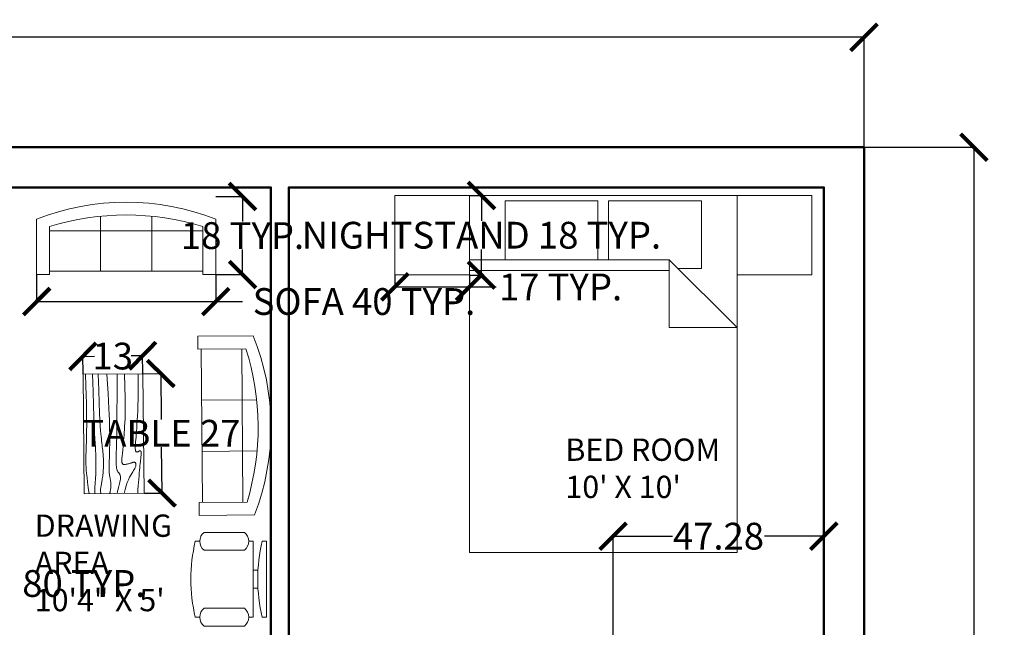
# Model space of a CAD drawing. Units: inches. Extents: x 9 to 573, y -373 to 44.
# Tile 5 of 5: x 329 to 550, y -92 to 44. Entities that reach past the tile are written whole.
import ezdxf

# ---------------------------------------------------------------- set-up
doc = ezdxf.new("R2010")
doc.units = ezdxf.units.IN
doc.header["$MEASUREMENT"] = 0
for name, color, linetype, lineweight in [('A-ANNO-DIMS', 2, 'Continuous', 18), ('A-AREA-IDEN', 7, 'Continuous', 25), ('A-FURN', 8, 'Continuous', 18), ('A-WALL', 7, 'Continuous', 50)]:
    doc.layers.add(name, color=color, linetype=linetype, lineweight=lineweight)
doc.styles.get("Standard").update_dxf_attribs({"font": 'arial.ttf'})
doc.dimstyles.get("Standard").update_dxf_attribs({"dimtxt": 6, "dimasz": 6, "dimexe": 0.18, "dimexo": 0.0625, "dimgap": 0.09, "dimtad": 0, "dimtih": 1, "dimtoh": 1, "dimdec": 0, "dimzin": 0, "dimdsep": 46, "dimlunit": 4, "dimtxsty": 'Standard', "dimblk": 'ARCHTICK', "dimcen": 0.09, "dimadec": 0, "dimazin": 0, "dimtfac": 1, "dimtdec": 0, "dimtofl": 0, "dimtmove": 0, "dimatfit": 3, "dimldrblk": 'ARCHTICK', "dimfxl": 1, "dimtolj": 1, "dimtzin": 0, "dimarcsym": 0})

# ---------------------------------------------------------------- blocks, each defined once
blk = doc.blocks.new('Chair - Desk')
for p, q in [((-8.5, 0), (-8.5, -1)), ((-8.5, 0), (8.5, 0)), ((8.5, 0), (8.5, -1)), ((-2, -3), (-2, -1.9355)), ((2, -1.9576), (2, -3)), ((-8.5, -3), (-8.5, -4)), ((-8.5, -3), (8.5, -3)), ((8.5, -3), (8.5, -4)), ((-10.5, -5), (-10.5, -14)), ((-6.5, -14), (-6.5, -5)), ((6.5, -5), (6.5, -14)), ((10.5, -14), (10.5, -5)), ((-8.5, -15), (-8.5, -16)), ((8.5, -15), (8.5, -16))]:
    blk.add_line(p, q)
for centre, radius, start, end in [((0, 34.625), 36.625, 256.5803, 283.4197), ((-8.5, -6.5), 2.5, 36.8699, 143.1301), ((8.5, -6.5), 2.5, 36.8699, 143.1301), ((-8.5, -12.5), 2.5, 216.8699, 323.1301), ((8.5, -12.5), 2.5, 216.8699, 323.1301), ((0, 19.625), 36.625, 256.5803, 283.4197)]:
    blk.add_arc(centre, radius, start, end)
blk = doc.blocks.new('Table - Rectangular Woodgrain 60 x 30 in.')
for p, q in [((0, 0), (0, -30)), ((60, 0), (0, 0)), ((60, -30), (60, 0)), ((0, -30), (60, -30))]:
    blk.add_line(p, q)
for points in [[(0, -2.4), (4.8155, -2.418), (9.0302, -2.4688), (12.709, -2.5477), (15.9167, -2.65), (18.7181, -2.7711), (21.1781, -2.9063), (23.3616, -3.0508), (25.3333, -3.2), (27.1477, -3.3495), (28.8172, -3.4958), (30.3437, -3.636), (31.7291, -3.7667), (32.9756, -3.8849), (34.0849, -3.9875), (35.059, -4.0714), (35.9, -4.1334), (36.6114, -4.1711), (37.2041, -4.1854), (37.6906, -4.1779), (38.0833, -4.15), (38.3948, -4.1034), (38.6375, -4.0396), (38.8239, -3.9602), (38.9666, -3.8667), (39.0764, -3.7608), (39.1573, -3.6448), (39.2116, -3.521), (39.2416, -3.3917), (39.2498, -3.2593), (39.2385, -3.1261), (39.21, -2.9944), (39.1666, -2.8667), (39.111, -2.7447), (39.0468, -2.6281), (38.978, -2.5163), (38.9083, -2.4083), (38.8418, -2.3035), (38.7823, -2.201), (38.7337, -2.1001), (38.7, -2), (38.6844, -1.9003), (38.6875, -1.8021), (38.7094, -1.707), (38.75, -1.6167), (38.8094, -1.5326), (38.8875, -1.4563), (38.9844, -1.3893), (39.1, -1.3333), (39.2351, -1.2896), (39.3937, -1.2583), (39.5804, -1.2396), (39.8, -1.2333), (40.057, -1.2396), (40.3562, -1.2583), (40.7023, -1.2896), (41.1, -1.3333), (41.5547, -1.3895), (42.0755, -1.4573), (42.6721, -1.5361), (43.3542, -1.625), (44.1316, -1.7233), (45.014, -1.8302), (46.0114, -1.9449), (47.1333, -2.0667), (48.3862, -2.1947), (49.7625, -2.3281), (51.2513, -2.4663), (52.8416, -2.6083), (54.5226, -2.7535), (56.2833, -2.9011), (58.1127, -3.0501), (60, -3.2)], [(0, -9.2), (6.5759, -9.0858), (11.9385, -9.0365), (16.2527, -9.0418), (19.6833, -9.0917), (22.3952, -9.1759), (24.5531, -9.2844), (26.322, -9.4069), (27.8666, -9.5333), (29.3241, -9.6553), (30.7203, -9.7719), (32.0532, -9.8837), (33.3208, -9.9917), (34.5213, -10.0965), (35.6526, -10.199), (36.7128, -10.2999), (37.7, -10.4), (38.6129, -10.4996), (39.4531, -10.5969), (40.223, -10.6895), (40.925, -10.775), (41.5613, -10.8512), (42.1344, -10.9156), (42.6465, -10.966), (43.1, -11), (43.4976, -11.0158), (43.8437, -11.0136), (44.143, -10.9942), (44.4, -10.9583), (44.6195, -10.9069), (44.8062, -10.8406), (44.9648, -10.7603), (45.1, -10.6667), (45.2155, -10.5598), (45.3114, -10.4365), (45.3871, -10.2929), (45.4416, -10.125), (45.4743, -9.929), (45.4844, -9.7011), (45.4709, -9.4371), (45.4333, -9.1333), (45.3716, -8.7883), (45.2896, -8.4104), (45.1919, -8.0107), (45.0833, -7.6), (44.9685, -7.1893), (44.8521, -6.7896), (44.7388, -6.4117), (44.6333, -6.0667), (44.54, -5.7628), (44.4614, -5.4979), (44.4001, -5.2675), (44.3583, -5.0667), (44.3384, -4.8909), (44.3427, -4.7354), (44.3736, -4.5956), (44.4333, -4.4667), (44.5236, -4.3453), (44.6427, -4.2333), (44.7884, -4.1339), (44.9583, -4.05), (45.1501, -3.9849), (45.3614, -3.9417), (45.59, -3.9234), (45.8333, -3.9333), (46.0915, -3.9749), (46.3734, -4.0531), (46.6906, -4.1736), (47.0542, -4.3417), (47.4756, -4.5629), (47.9661, -4.8427), (48.5372, -5.1866), (49.2, -5.6), (49.9676, -6.0844), (50.8594, -6.625), (51.8965, -7.2031), (53.1, -7.8), (54.491, -8.3969), (56.0906, -8.975), (57.9199, -9.5156), (60, -10)], [(0, -12.8), (5.1847, -12.9322), (9.6213, -13.0323), (13.3963, -13.1059), (16.5958, -13.1583), (19.3063, -13.1952), (21.614, -13.2219), (23.6054, -13.2439), (25.3666, -13.2667), (26.9728, -13.2947), (28.4531, -13.3281), (29.8256, -13.3663), (31.1083, -13.4083), (32.3191, -13.4535), (33.476, -13.501), (34.597, -13.5501), (35.7, -13.6), (36.7984, -13.6497), (37.8875, -13.6979), (38.9578, -13.743), (40, -13.7833), (41.0047, -13.8174), (41.9625, -13.8438), (42.864, -13.8607), (43.7, -13.8667), (44.4631, -13.8604), (45.1552, -13.8417), (45.7801, -13.8104), (46.3416, -13.7667), (46.8439, -13.7104), (47.2906, -13.6417), (47.6858, -13.5604), (48.0333, -13.4667), (48.3375, -13.3608), (48.6042, -13.2448), (48.8396, -13.121), (49.05, -12.9917), (49.2417, -12.8593), (49.4208, -12.7261), (49.5937, -12.5944), (49.7667, -12.4667), (49.9452, -12.3451), (50.1323, -12.2313), (50.3303, -12.1268), (50.5416, -12.0333), (50.7686, -11.9524), (51.0135, -11.8854), (51.2788, -11.8341), (51.5666, -11.8), (51.8785, -11.7843), (52.2116, -11.7865), (52.562, -11.8059), (52.926, -11.8417), (53.2998, -11.8931), (53.6795, -11.9594), (54.0614, -12.0397), (54.4416, -12.1333), (54.8223, -12.2401), (55.2293, -12.3625), (55.6942, -12.5037), (56.2489, -12.6667), (56.9251, -12.8547), (57.7545, -13.0708), (58.7689, -13.3182), (60, -13.6)], [(0, -18), (5.124, -17.7273), (9.6609, -17.5057), (13.6705, -17.3303), (17.2125, -17.1958), (20.3467, -17.0973), (23.1328, -17.0297), (25.6307, -16.9878), (27.9, -16.9667), (29.9928, -16.9617), (31.9302, -16.9703), (33.7254, -16.9907), (35.3917, -17.0208), (36.9423, -17.0588), (38.3906, -17.1026), (39.7499, -17.1503), (41.0333, -17.2), (42.2519, -17.2496), (43.4073, -17.2969), (44.4986, -17.3395), (45.525, -17.375), (46.4858, -17.4012), (47.3802, -17.4156), (48.2074, -17.416), (48.9667, -17.4), (49.6583, -17.3662), (50.2872, -17.3167), (50.8595, -17.2547), (51.3812, -17.1833), (51.8584, -17.1057), (52.2971, -17.025), (52.7034, -16.9443), (53.0833, -16.8667), (53.443, -16.7951), (53.789, -16.7313), (54.128, -16.6768), (54.4666, -16.6334), (54.8115, -16.6024), (55.1693, -16.5854), (55.5465, -16.5841), (55.95, -16.6), (56.3828, -16.6337), (56.8346, -16.6823), (57.2915, -16.7418), (57.7396, -16.8084), (58.165, -16.878), (58.5539, -16.9469), (58.8924, -17.0111), (59.1666, -17.0667), (59.3679, -17.1107), (59.5078, -17.1438), (59.6032, -17.1675), (59.6708, -17.1833), (59.7275, -17.193), (59.7901, -17.1979), (59.8753, -17.1998), (60, -17.2)], [(0, -22.4), (8.0098, -22.2501), (14.4094, -22.1011), (19.4168, -21.9535), (23.25, -21.8083), (26.1269, -21.6663), (28.2656, -21.5281), (29.884, -21.3947), (31.2, -21.2667), (32.3967, -21.1448), (33.5172, -21.0292), (34.5697, -20.9198), (35.5625, -20.8167), (36.5037, -20.7198), (37.4015, -20.6292), (38.2642, -20.5448), (39.1, -20.4667), (39.9164, -20.3951), (40.7187, -20.3313), (41.5117, -20.2768), (42.3, -20.2333), (43.0883, -20.2024), (43.8812, -20.1854), (44.6836, -20.1841), (45.5, -20.2), (46.3328, -20.234), (47.1747, -20.2844), (48.0163, -20.3488), (48.8479, -20.425), (49.66, -20.5106), (50.4429, -20.6031), (51.1872, -20.7004), (51.8833, -20.8), (52.5246, -20.8999), (53.1166, -20.9995), (53.6681, -21.0983), (54.1875, -21.1958), (54.6834, -21.2919), (55.1646, -21.3859), (55.6394, -21.4777), (56.1167, -21.5667), (56.6028, -21.6515), (57.0961, -21.7266), (57.5929, -21.7852), (58.0896, -21.8208), (58.5823, -21.8268), (59.0674, -21.7964), (59.5412, -21.723), (60, -21.6)], [(0, -25.2), (8.6355, -25.0504), (15.7026, -24.9031), (21.4049, -24.7606), (25.9458, -24.625), (29.529, -24.4988), (32.3578, -24.3844), (34.6359, -24.284), (36.5667, -24.2), (38.3213, -24.1341), (39.9417, -24.0854), (41.437, -24.0523), (42.8167, -24.0333), (44.0901, -24.0268), (45.2667, -24.0313), (46.3557, -24.0451), (47.3667, -24.0667), (48.309, -24.0947), (49.1928, -24.1287), (50.0284, -24.168), (50.826, -24.2125), (51.5959, -24.2617), (52.3483, -24.3151), (53.0935, -24.3725), (53.8417, -24.4334), (54.6009, -24.497), (55.3699, -24.561), (56.1454, -24.6226), (56.9239, -24.6792), (57.7021, -24.7279), (58.4764, -24.7662), (59.2435, -24.7911), (60, -24.8)], [(0, -28.8), (5.6867, -28.6681), (10.45, -28.5698), (14.407, -28.5012), (17.675, -28.4584), (20.3711, -28.4374), (22.6125, -28.4344), (24.5164, -28.4455), (26.2, -28.4667), (27.762, -28.4947), (29.2276, -28.5281), (30.6033, -28.5663), (31.8958, -28.6084), (33.1118, -28.6535), (34.2578, -28.7011), (35.3405, -28.7501), (36.3666, -28.8), (37.3443, -28.8497), (38.288, -28.8974), (39.2137, -28.9412), (40.1375, -28.9792), (41.0753, -29.0093), (42.0432, -29.0297), (43.0572, -29.0384), (44.1333, -29.0333), (45.2936, -29.0114), (46.5843, -28.9641), (48.0579, -28.8816), (49.7666, -28.7542), (51.7629, -28.5721), (54.0989, -28.3255), (56.8272, -28.0048), (60, -27.6)]]:
    blk.add_lwpolyline(points)
blk = doc.blocks.new('Bed - Queen')
for p, q in [((0, -80.00003), (0, 0)), ((0, 0), (59.99999, 0)), ((59.99999, 0), (59.99999, -80.00003)), ((7.99999, -1.2), (28.79998, -1.2)), ((7.99999, -14.4), (7.99999, -1.2)), ((28.79998, -1.2), (28.79998, -14.4)), ((31.19999, -1.2), (51.99999, -1.2)), ((31.19999, -14.4), (31.19999, -1.2)), ((51.99999, -1.2), (51.99999, -16.4)), ((0, -14.4), (44.8, -14.4)), ((59.99999, -29.6), (44.8, -14.4)), ((44.8, -14.4), (44.8, -29.6)), ((44.8, -16.8), (0, -16.8)), ((51.99999, -16.4), (46.79936, -16.4)), ((44.8, -29.6), (59.99999, -29.6)), ((59.99999, -80.00003), (0, -80.00003))]:
    blk.add_line(p, q)
blk = doc.blocks.new('Sofa - Roundback 7 ft.')
for p, q in [((-12.00002, -32.4421), (-12.00003, -6.5971)), ((11.99997, -32.4421), (11.99998, -6.5971)), ((-36.000027, -34), (-36.000027, -11.4696)), ((-35.999844, -13.3819), (35.9998, -13.3819)), ((35.99998, -34), (35.99998, -11.4696)), ((-36.000027, -32.4421), (35.99998, -32.4421))]:
    blk.add_line(p, q)
for points in [[(-36.000027, -34), (-42.000027, -34), (-42.000027, -8)], [(41.99998, -8), (41.99998, -34), (35.99998, -34)]]:
    blk.add_lwpolyline(points)
for centre, radius, start, end in [((0, -114.25), 114.25, 68.43141, 111.5686), ((-0.00001, -127.1968), 121.1968, 72.72033, 107.2797)]:
    blk.add_arc(centre, radius, start, end)
blk = doc.blocks.new('BEDSIDE-TABLE')
blk.add_lwpolyline([(0, 17.82), (16.74, 17.82), (16.74, 0), (0, 0)], close=True)
blk = doc.blocks.new('_ArchTick')
at = {"color": 0, "linetype": 'ByBlock', "const_width": 0.15}
blk.add_lwpolyline([(-0.5, -0.5), (0.5, 0.5)], dxfattribs=at)
blk = doc.blocks.new('*D30')
at = {"layer": 'A-ANNO-DIMS', "color": 0, "lineweight": -2, "transparency": 16777216}
for p, q in [((193.52, -70), (193.52, -82.12)), ((273.52, -70), (273.52, -82.12)), ((193.52, -81.94), (273.52, -81.94)), ((273.52, -81.94), (279.52, -81.94))]:
    blk.add_line(p, q, dxfattribs=at)
at = {"layer": 'Defpoints', "color": 0, "transparency": 16777216}
for p in [(193.52, -69.94), (273.52, -69.94), (273.52, -81.94)]:
    blk.add_point(p, dxfattribs=at)
at = {"layer": 'A-ANNO-DIMS', "color": 0, "lineweight": -2, "transparency": 16777216, "xscale": 6, "yscale": 6, "zscale": 6, "rotation": 180}
blk.add_blockref('_ArchTick', (193.52, -81.94), dxfattribs=at)
at = {"layer": 'A-ANNO-DIMS', "color": 0, "lineweight": -2, "transparency": 16777216, "xscale": 6, "yscale": 6, "zscale": 6}
blk.add_blockref('_ArchTick', (273.52, -81.94), dxfattribs=at)
at = {"layer": 'A-ANNO-DIMS', "color": 0, "transparency": 16777216, "insert": (320.05, -81.94), "char_height": 6, "attachment_point": 5}
blk.add_mtext('\\A1;QUEEN BED 80 TYP.', dxfattribs=at)
blk = doc.blocks.new('*D32')
at = {"layer": 'A-ANNO-DIMS', "color": 0, "lineweight": -2, "transparency": 16777216}
for p, q in [((430.12, 5.01), (432.91, 5.01)), ((432.73, 5.01), (432.73, -0.71)), ((432.73, -12.82), (432.73, -7.1)), ((430.12, -12.82), (432.91, -12.82))]:
    blk.add_line(p, q, dxfattribs=at)
at = {"layer": 'Defpoints', "color": 0, "transparency": 16777216}
for p in [(430.05, 5.01), (432.73, 5.01), (430.05, -12.82)]:
    blk.add_point(p, dxfattribs=at)
at = {"layer": 'A-ANNO-DIMS', "color": 0, "lineweight": -2, "transparency": 16777216, "xscale": 6, "yscale": 6, "zscale": 6}
for p, rotation in [((432.73, 5.01), 90), ((432.73, -12.82), 270)]:
    blk.add_blockref('_ArchTick', p, dxfattribs=dict(at, rotation=rotation))
at = {"layer": 'A-ANNO-DIMS', "color": 0, "transparency": 16777216, "insert": (432.73, -3.9), "char_height": 6, "attachment_point": 5}
blk.add_mtext('\\A1;NIGHTSTAND 18 TYP.', dxfattribs=at)
blk = doc.blocks.new('*D33')
at = {"layer": 'A-ANNO-DIMS', "color": 0, "lineweight": -2, "transparency": 16777216}
for p, q in [((413.31, -12.88), (413.31, -15.67)), ((430.05, -12.88), (430.05, -15.67)), ((413.31, -15.49), (430.05, -15.49)), ((430.05, -15.49), (436.05, -15.49))]:
    blk.add_line(p, q, dxfattribs=at)
at = {"layer": 'Defpoints', "color": 0, "transparency": 16777216}
for p in [(413.31, -12.82), (430.05, -12.82), (430.05, -15.49)]:
    blk.add_point(p, dxfattribs=at)
at = {"layer": 'A-ANNO-DIMS', "color": 0, "lineweight": -2, "transparency": 16777216, "xscale": 6, "yscale": 6, "zscale": 6, "rotation": 180}
blk.add_blockref('_ArchTick', (413.31, -15.49), dxfattribs=at)
at = {"layer": 'A-ANNO-DIMS', "color": 0, "lineweight": -2, "transparency": 16777216, "xscale": 6, "yscale": 6, "zscale": 6}
blk.add_blockref('_ArchTick', (430.05, -15.49), dxfattribs=at)
at = {"layer": 'A-ANNO-DIMS', "color": 0, "transparency": 16777216, "insert": (450.47, -15.49), "char_height": 6, "attachment_point": 5}
blk.add_mtext('\\A1;17 TYP.', dxfattribs=at)
blk = doc.blocks.new('*D44')
at = {"layer": 'A-ANNO-DIMS', "color": 0, "lineweight": -2, "transparency": 16777216}
for p, q in [((332.98, -12.8), (332.98, -18.94)), ((373.13, -12.8), (373.13, -18.94)), ((332.98, -18.76), (373.13, -18.76)), ((373.13, -18.76), (379.13, -18.76))]:
    blk.add_line(p, q, dxfattribs=at)
at = {"layer": 'Defpoints', "color": 0, "transparency": 16777216}
for p in [(332.98, -12.74), (373.13, -12.74), (373.13, -18.76)]:
    blk.add_point(p, dxfattribs=at)
at = {"layer": 'A-ANNO-DIMS', "color": 0, "lineweight": -2, "transparency": 16777216, "xscale": 6, "yscale": 6, "zscale": 6, "rotation": 180}
blk.add_blockref('_ArchTick', (332.98, -18.76), dxfattribs=at)
at = {"layer": 'A-ANNO-DIMS', "color": 0, "lineweight": -2, "transparency": 16777216, "xscale": 6, "yscale": 6, "zscale": 6}
blk.add_blockref('_ArchTick', (373.13, -18.76), dxfattribs=at)
at = {"layer": 'A-ANNO-DIMS', "color": 0, "transparency": 16777216, "insert": (406.38, -18.76), "char_height": 6, "attachment_point": 5}
blk.add_mtext('\\A1;SOFA 40 TYP.', dxfattribs=at)
blk = doc.blocks.new('*D45')
at = {"layer": 'A-ANNO-DIMS', "color": 0, "lineweight": -2, "transparency": 16777216}
for p, q in [((373.19, 4.78), (379.33, 4.78)), ((379.15, 4.78), (379.15, -0.83)), ((379.15, -12.74), (379.15, -7.13)), ((373.19, -12.74), (379.33, -12.74))]:
    blk.add_line(p, q, dxfattribs=at)
at = {"layer": 'Defpoints', "color": 0, "transparency": 16777216}
for p in [(373.13, 4.78), (379.15, 4.78), (373.13, -12.74)]:
    blk.add_point(p, dxfattribs=at)
at = {"layer": 'A-ANNO-DIMS', "color": 0, "lineweight": -2, "transparency": 16777216, "xscale": 6, "yscale": 6, "zscale": 6}
for p, rotation in [((379.15, 4.78), 90), ((379.15, -12.74), 270)]:
    blk.add_blockref('_ArchTick', p, dxfattribs=dict(at, rotation=rotation))
at = {"layer": 'A-ANNO-DIMS', "color": 0, "transparency": 16777216, "insert": (379.15, -3.98), "char_height": 6, "attachment_point": 5}
blk.add_mtext('\\A1;18 TYP.', dxfattribs=at)
blk = doc.blocks.new('*D48')
at = {"layer": 'A-ANNO-DIMS', "color": 0, "lineweight": -2, "transparency": 16777216}
for p, q in [((356.85, -34.93), (360.99, -34.88)), ((360.81, -34.89), (360.92, -45.19)), ((361.1, -61.7), (360.99, -51.4)), ((357.14, -61.74), (361.28, -61.69))]:
    blk.add_line(p, q, dxfattribs=at)
at = {"layer": 'Defpoints', "color": 0, "transparency": 16777216}
for p in [(356.79, -34.93), (357.08, -61.74), (361.1, -61.7)]:
    blk.add_point(p, dxfattribs=at)
at = {"layer": 'A-ANNO-DIMS', "color": 0, "lineweight": -2, "transparency": 16777216, "xscale": 6, "yscale": 6, "zscale": 6}
for p, rotation in [((360.81, -34.89), 90.61221498216747), ((361.1, -61.7), 270.6122149821675)]:
    blk.add_blockref('_ArchTick', p, dxfattribs=dict(at, rotation=rotation))
at = {"layer": 'A-ANNO-DIMS', "color": 0, "transparency": 16777216, "insert": (360.96, -48.29), "char_height": 6, "attachment_point": 5}
blk.add_mtext('\\A1;TABLE 27', dxfattribs=at)
blk = doc.blocks.new('*D49')
at = {"layer": 'A-ANNO-DIMS', "color": 0, "lineweight": -2, "transparency": 16777216}
for p, q in [((343.38, -35.01), (343.34, -30.87)), ((356.75, -30.91), (354.15, -30.93)), ((356.79, -34.87), (356.75, -30.73)), ((343.34, -31.05), (345.94, -31.02))]:
    blk.add_line(p, q, dxfattribs=at)
at = {"layer": 'Defpoints', "color": 0, "transparency": 16777216}
for p in [(356.75, -30.91), (343.39, -35.07), (356.79, -34.93)]:
    blk.add_point(p, dxfattribs=at)
at = {"layer": 'A-ANNO-DIMS', "color": 0, "lineweight": -2, "transparency": 16777216, "xscale": 6, "yscale": 6, "zscale": 6}
for p, rotation in [((343.34, -31.05), 180.6122149821674), ((356.75, -30.91), 0.6122149821674369)]:
    blk.add_blockref('_ArchTick', p, dxfattribs=dict(at, rotation=rotation))
at = {"layer": 'A-ANNO-DIMS', "color": 0, "transparency": 16777216, "insert": (350.05, -30.98), "char_height": 6, "attachment_point": 5}
blk.add_mtext('\\A1;13', dxfattribs=at)
blk = doc.blocks.new('*D58')
at = {"layer": 'A-ANNO-DIMS', "color": 0, "lineweight": -2, "transparency": 16777216}
for p, q in [((38.52, 15.87), (38.52, 40.63)), ((38.52, 40.45), (271.69, 40.45)), ((518.52, 40.45), (285.35, 40.45)), ((518.52, 15.87), (518.52, 40.63))]:
    blk.add_line(p, q, dxfattribs=at)
at = {"layer": 'Defpoints', "color": 0, "transparency": 16777216}
for p in [(518.52, 40.45), (38.52, 15.8), (518.52, 15.8)]:
    blk.add_point(p, dxfattribs=at)
at = {"layer": 'A-ANNO-DIMS', "color": 0, "lineweight": -2, "transparency": 16777216, "xscale": 6, "yscale": 6, "zscale": 6, "rotation": 180}
blk.add_blockref('_ArchTick', (38.52, 40.45), dxfattribs=at)
at = {"layer": 'A-ANNO-DIMS', "color": 0, "lineweight": -2, "transparency": 16777216, "xscale": 6, "yscale": 6, "zscale": 6}
blk.add_blockref('_ArchTick', (518.52, 40.45), dxfattribs=at)
at = {"layer": 'A-ANNO-DIMS', "color": 0, "transparency": 16777216, "insert": (278.52, 40.45), "char_height": 6, "attachment_point": 5}
blk.add_mtext('\\A1;480', dxfattribs=at)
blk = doc.blocks.new('*D59')
at = {"layer": 'A-ANNO-DIMS', "color": 0, "lineweight": -2, "transparency": 16777216}
for p, q in [((518.58, 15.8), (543.35, 15.8)), ((543.17, 15.8), (543.17, -161.04)), ((543.17, -344.2), (543.17, -167.35)), ((518.58, -344.2), (543.35, -344.2))]:
    blk.add_line(p, q, dxfattribs=at)
at = {"layer": 'Defpoints', "color": 0, "transparency": 16777216}
for p in [(518.52, 15.8), (518.52, -344.2), (543.17, -344.2)]:
    blk.add_point(p, dxfattribs=at)
at = {"layer": 'A-ANNO-DIMS', "color": 0, "lineweight": -2, "transparency": 16777216, "xscale": 6, "yscale": 6, "zscale": 6}
for p, rotation in [((543.17, 15.8), 90), ((543.17, -344.2), 270)]:
    blk.add_blockref('_ArchTick', p, dxfattribs=dict(at, rotation=rotation))
at = {"layer": 'A-ANNO-DIMS', "color": 0, "transparency": 16777216, "insert": (543.17, -164.2), "char_height": 6, "attachment_point": 5}
blk.add_mtext('\\A1;360', dxfattribs=at)
blk = doc.blocks.new('*D92')
at = {"layer": 'A-ANNO-DIMS', "color": 0, "lineweight": -2, "transparency": 16777216}
for p, q in [((462.24, -95.93), (462.24, -71.16)), ((462.24, -71.34), (475.54, -71.34)), ((509.52, -71.34), (496.22, -71.34)), ((509.52, -95.93), (509.52, -71.16))]:
    blk.add_line(p, q, dxfattribs=at)
at = {"layer": 'Defpoints', "color": 0, "transparency": 16777216}
for p in [(509.52, -71.34), (462.24, -95.99), (509.52, -95.99)]:
    blk.add_point(p, dxfattribs=at)
at = {"layer": 'A-ANNO-DIMS', "color": 0, "lineweight": -2, "transparency": 16777216, "xscale": 6, "yscale": 6, "zscale": 6, "rotation": 180}
blk.add_blockref('_ArchTick', (462.24, -71.34), dxfattribs=at)
at = {"layer": 'A-ANNO-DIMS', "color": 0, "lineweight": -2, "transparency": 16777216, "xscale": 6, "yscale": 6, "zscale": 6}
blk.add_blockref('_ArchTick', (509.52, -71.34), dxfattribs=at)
at = {"layer": 'A-ANNO-DIMS', "color": 0, "transparency": 16777216, "insert": (485.88, -71.34), "char_height": 6, "attachment_point": 5}
blk.add_mtext('\\A1;47.28', dxfattribs=at)

msp = doc.modelspace()

# ---------------------------------------------------------------- linework, layer by layer
at = {"layer": 'A-WALL'}
msp.add_lwpolyline([(329.5169, -215.1966), (329.5169, -335.1966), (509.5169, -335.1966), (518.5169, -335.1966), (518.5169, -344.1966), (38.5169, -344.1966), (38.5169, 15.8034), (518.5169, 15.8034), (518.5169, -117.1966), (450.7536, -117.1966), (450.7536, -140.1966), (446.7536, -140.1966), (446.7536, -117.1966), (431.5169, -117.1966), (431.5169, -113.1966), (509.5169, -113.1966), (509.5169, 6.8034), (389.5169, 6.8034), (389.5169, -113.1966), (395.5169, -113.1966), (395.5169, -117.1966), (385.5169, -117.1966), (385.5169, 6.8034), (325.5169, 6.8034)], dxfattribs=at)

# ---------------------------------------------------------------- block references
at = {"layer": 'A-FURN', "xscale": 0.4779142578925423, "yscale": 0.4779142578925423, "zscale": 0.4779142578925423}
msp.add_blockref('Sofa - Roundback 7 ft.', (353.0545, 3.5085), dxfattribs=at)
at = {"layer": 'A-FURN'}
for name, p in [('BEDSIDE-TABLE', (413.3124, -12.816)), ('Bed - Queen', (430.0545, 5.0085)), ('BEDSIDE-TABLE', (490.054, -12.816))]:
    msp.add_blockref(name, p, dxfattribs=at)
for name, p, xscale, yscale, zscale, rotation in [('Sofa - Roundback 7 ft.', (385.5169, -46.4915), -0.4779142578925423, 0.4779142578925423, 0.4779142578925423, 270.4087265423498), ('Table - Rectangular Woodgrain 60 x 30 in.', (356.7907, -34.9287), 0.4468643707391663, 0.4468643707391663, 0.4468643707391663, 270.6122149821675)]:
    msp.add_blockref(name, p, dxfattribs=dict(at, xscale=xscale, yscale=yscale, zscale=zscale, rotation=rotation))
at = {"layer": 'A-FURN', "rotation": 270}
msp.add_blockref('Chair - Desk', (384.5545, -80.9915), dxfattribs=at)

# ---------------------------------------------------------------- texts
at = {"layer": 'A-AREA-IDEN', "char_height": 5, "attachment_point": 1}
for s, width, insert in [("BED ROOM \\P10' X 10'", 57.999995, (451.5545, -49.4638)), ('DRAWING AREA \\P10\'4" X 5\'', 48.148745, (332.5545, -66.4915))]:
    msp.add_mtext_dynamic_manual_height_columns(s, width=width, gutter_width=1, heights=[0], dxfattribs=dict(at, insert=insert))

# ---------------------------------------------------------------- dimensions: what is measured, and where the dimension line sits
at = {"layer": 'A-ANNO-DIMS'}
for base, p1, p2, override, picture, middle in [((518.5169, 40.4534), (38.5169, 15.8034), (518.5169, 15.8034), {"dimdec": 0, "dimlfac": 1, "dimrnd": 0, "dimzin": 0, "dimdsep": 46, "dimlunit": 2}, '*D58', (278.5169, 40.4534)), ((509.5169, -71.3415), (462.2364, -95.9915), (509.5169, -95.9915), {"dimdec": 2, "dimlfac": 1, "dimrnd": 0, "dimzin": 0, "dimdsep": 46, "dimlunit": 2}, '*D92', (485.8766, -71.3415))]:
    dim = msp.add_linear_dim(base=base, p1=p1, p2=p2, dimstyle='Standard', override=override, dxfattribs=at)
    dim.commit()
    dim.dimension.update_dxf_attribs({"geometry": picture, "text_midpoint": middle})
for base, p1, p2, angle, picture, middle in [((543.1669, -344.1966), (518.5169, 15.8034), (518.5169, -344.1966), 270, '*D59', (543.1669, -164.1966)), ((356.7477, -30.9072), (343.3855, -35.072), (356.7907, -34.9287), 0.612215, '*D49', (350.0451, -30.9788))]:
    dim = msp.add_linear_dim(base=base, p1=p1, p2=p2, angle=angle, dimstyle='Standard', override={"dimdec": 0, "dimlfac": 1, "dimrnd": 0, "dimzin": 0, "dimdsep": 46, "dimlunit": 2}, dxfattribs=at)
    dim.commit()
    dim.dimension.update_dxf_attribs({"geometry": picture, "text_midpoint": middle})
for base, p1, p2, angle, text, picture, middle in [((432.7282, 5.0085), (430.0545, -12.8165), (430.0545, 5.0085), 90, 'NIGHTSTAND <> TYP.', '*D32', (432.7282, -3.904)), ((379.1486, 4.7829), (373.1269, -12.7406), (373.1269, 4.7829), 90, '<> TYP.', '*D45', (379.1486, -3.9788)), ((361.0987, -61.6961), (356.7907, -34.9287), (357.0772, -61.7391), 270.612215, 'TABLE <>', '*D48', (360.9555, -48.2909))]:
    dim = msp.add_linear_dim(base=base, p1=p1, p2=p2, angle=angle, text=text, dimstyle='Standard', override={"dimdec": 0, "dimlfac": 1, "dimrnd": 0, "dimzin": 0, "dimdsep": 46, "dimlunit": 2}, dxfattribs=at)
    dim.commit()
    dim.dimension.update_dxf_attribs({"geometry": picture, "text_midpoint": middle})
for base, p1, p2, text, picture, middle in [((373.1269, -18.7623), (332.9821, -12.7406), (373.1269, -12.7406), 'SOFA <> TYP.', '*D44', (406.3806, -18.7623)), ((430.0545, -15.4902), (413.3129, -12.8165), (430.0545, -12.8165), '<> TYP.', '*D33', (450.4651, -15.4902)), ((273.5169, -81.9382), (193.5168, -69.9382), (273.5169, -69.9382), 'QUEEN BED <> TYP.', '*D30', (320.0537, -81.9382))]:
    dim = msp.add_linear_dim(base=base, p1=p1, p2=p2, text=text, dimstyle='Standard', override={"dimdec": 0, "dimlfac": 1, "dimrnd": 0, "dimzin": 0, "dimdsep": 46, "dimlunit": 2}, dxfattribs=at)
    dim.commit()
    dim.dimension.update_dxf_attribs({"geometry": picture, "text_midpoint": middle})

doc.saveas('drawing.dxf')
